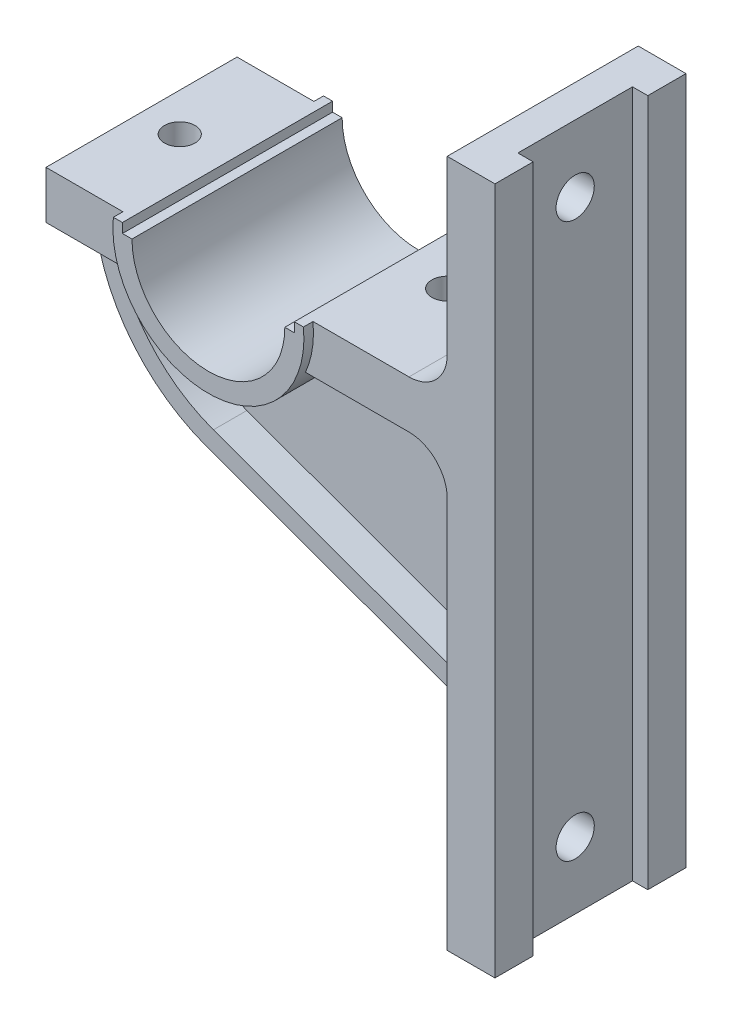
from build123d import *

# Parameters (mm, degrees)
BRACKET_BODY_DEPTH     = 50
POCKET_SKETCH_W        = 8
POCKET_SKETCH_H        = 60
POCKET_60X30_DEPTH     = 433.810582126
RAISED_PAD_SKETCH_R    = 25
RAISED_PAD_5MM_DEPTH   = 5
PAD_HOLE_SKETCH_R      = 10
PAD_HOLES_DEPTH        = 328.146756059
MOUNTING_HOLE_SKETCH_R = 7.25
MOUNTING_HOLES_DEPTH   = 25
THROUGH_HOLE_SKETCH_R  = 8
THROUGH_HOLES_16_DEPTH = 20
SADDLE_BLOCK_DEPTH     = 55
PIPE_SADDLE_CUT_DEPTH  = 55
SUPPORT_ARM_DEPTH      = 25
SUPPORT_WEB_15MM_DEPTH = 7.5


with BuildPart() as part:
    # Bracket Profile Sketch → Bracket Body (new, symmetric)
    with BuildSketch(Plane.XY):
        with BuildLine():
            Line((0, 110), (0, -250))
            Line((0, -250), (-25, -250))
            Line((-25, -250), (-25, -45))
            ThreePointArc((-25, -45), (-30.857864376, -30.857864376), (-45, -25))
            Line((-45, -25), (-235, -25))
            Line((-235, -25), (-235, 0))
            Line((-235, 0), (-45, 0))
            ThreePointArc((-45, 0), (-30.857864376, 5.857864376), (-25, 20))
            Line((-25, 20), (-25, 110))
            Line((-25, 110), (0, 110))
        make_face()
    extrude(amount=BRACKET_BODY_DEPTH, both=True)

    # Pocket Sketch → Pocket 60x30 (cut, through all)
    with BuildSketch(Plane(origin=(0, 110, 0), x_dir=(1, 0, 0), z_dir=(0, 1, 0))):
        with Locations((-4, 0)):
            Rectangle(POCKET_SKETCH_W, POCKET_SKETCH_H)
    extrude(amount=-POCKET_60X30_DEPTH, mode=Mode.SUBTRACT)

    # Raised Pad Sketch → Raised Pad 5mm (add)
    with BuildSketch(Plane.ZY.offset(25)):
        with Locations(Location((0, 75, 0), (0, 0, 90))):
            Circle(RAISED_PAD_SKETCH_R)
        with Locations(Location((0, -215, 0), (0, 0, 180))):
            Circle(RAISED_PAD_SKETCH_R)
    extrude(amount=RAISED_PAD_5MM_DEPTH)

    # Pad Hole Sketch → Pad Holes (cut, through all)
    with BuildSketch(Plane.ZY.offset(30)):
        with Locations(Location((0, 75, 0), (0, 0, 270))):
            Circle(PAD_HOLE_SKETCH_R)
        with Locations(Location((0, -215, 0), (0, 0, 270))):
            Circle(PAD_HOLE_SKETCH_R)
    extrude(amount=-PAD_HOLES_DEPTH, mode=Mode.SUBTRACT)

    # Mounting Hole Sketch → Mounting Holes (cut)
    with BuildSketch(Plane(origin=(0, 0, 0), x_dir=(1, 0, 0), z_dir=(0, 1, 0))):
        with Locations(Location((-75, 0, 0), (0, 0, 270))):
            Circle(MOUNTING_HOLE_SKETCH_R)
        with Locations(Location((-215, 0, 0), (0, 0, 270))):
            Circle(MOUNTING_HOLE_SKETCH_R)
    extrude(amount=-MOUNTING_HOLES_DEPTH, mode=Mode.SUBTRACT)

    # Through Hole Sketch → Through Holes Ø16 (cut)
    with BuildSketch(Plane(origin=(0, 0, 0), x_dir=(1, 0, 0), z_dir=(0, 1, 0))):
        with Locations(Location((-75, 0, 0), (0, 0, 270))):
            Circle(THROUGH_HOLE_SKETCH_R)
        with Locations(Location((-215, 0, 0), (0, 0, 270))):
            Circle(THROUGH_HOLE_SKETCH_R)
    extrude(amount=-THROUGH_HOLES_16_DEPTH, mode=Mode.SUBTRACT)

    # Saddle Block Sketch → Saddle Block (add, symmetric)
    with BuildSketch(Plane.XY):
        with BuildLine():
            Line((-194.749371855, 0), (-95.250628145, 0))
            ThreePointArc((-95.250628145, 0), (-145, -55), (-194.749371855, 0))
        make_face()
    extrude(amount=SADDLE_BLOCK_DEPTH, both=True)

    # Pipe Saddle Cut Sketch → Pipe Saddle Cut (cut, symmetric)
    with BuildSketch(Plane.XY):
        with BuildLine():
            Line((-190, 0), (-100, 0))
            Line((-100, 0), (-100, -5))
            Line((-100, -5), (-105, -5))
            ThreePointArc((-105, -5), (-145, -45), (-185, -5))
            Line((-185, -5), (-190, -5))
            Line((-190, -5), (-190, 0))
        make_face()
    extrude(amount=PIPE_SADDLE_CUT_DEPTH, both=True, mode=Mode.SUBTRACT)

    # Support Arm Sketch → Support Arm (add, symmetric)
    with BuildSketch(Plane.XY):
        with BuildLine():
            Line((-41.449496417, -158.46530057), (-175.781812899, -109.572335871))
            ThreePointArc((-175.781812899, -109.572335871), (-218.723683986, -76.621879272), (-235, -25))
            Line((-235, -25), (-219.833147735, -25))
            ThreePointArc((-219.833147735, -25), (-223.484631452, -26.584349745), (-224.822024251, -30.333333333))
            ThreePointArc((-224.822024251, -30.333333333), (-208.965317539, -73.046208509), (-172.361611466, -100.175409663))
            Line((-172.361611466, -100.175409663), (-42.446261863, -147.460729893))
            ThreePointArc((-42.446261863, -147.460729893), (-30.543506327, -145.893702398), (-25, -135.244725822))
            Line((-25, -135.244725822), (-25, -181.95761609))
            ThreePointArc((-25, -181.95761609), (-29.521198893, -167.618205181), (-41.449496417, -158.46530057))
        make_face()
    extrude(amount=SUPPORT_ARM_DEPTH, both=True)

    # Support Web Sketch → Support Web 15mm (add, symmetric)
    with BuildSketch(Plane.XY):
        with BuildLine():
            Line((-25, -45), (-25, -135.244725822))
            ThreePointArc((-25, -135.244725822), (-30.543506327, -145.893702398), (-42.446261863, -147.460729893))
            Line((-42.446261863, -147.460729893), (-172.361611466, -100.175409663))
            ThreePointArc((-172.361611466, -100.175409663), (-208.965317539, -73.046208509), (-224.822024251, -30.333333333))
            ThreePointArc((-224.822024251, -30.333333333), (-223.484631452, -26.584349745), (-219.833147735, -25))
            Line((-219.833147735, -25), (-190.82575695, -25))
            ThreePointArc((-190.82575695, -25), (-145, -55), (-99.17424305, -25))
            Line((-99.17424305, -25), (-45, -25))
            ThreePointArc((-45, -25), (-30.857864376, -30.857864376), (-25, -45))
        make_face()
    extrude(amount=SUPPORT_WEB_15MM_DEPTH, both=True)


solid = part.part
